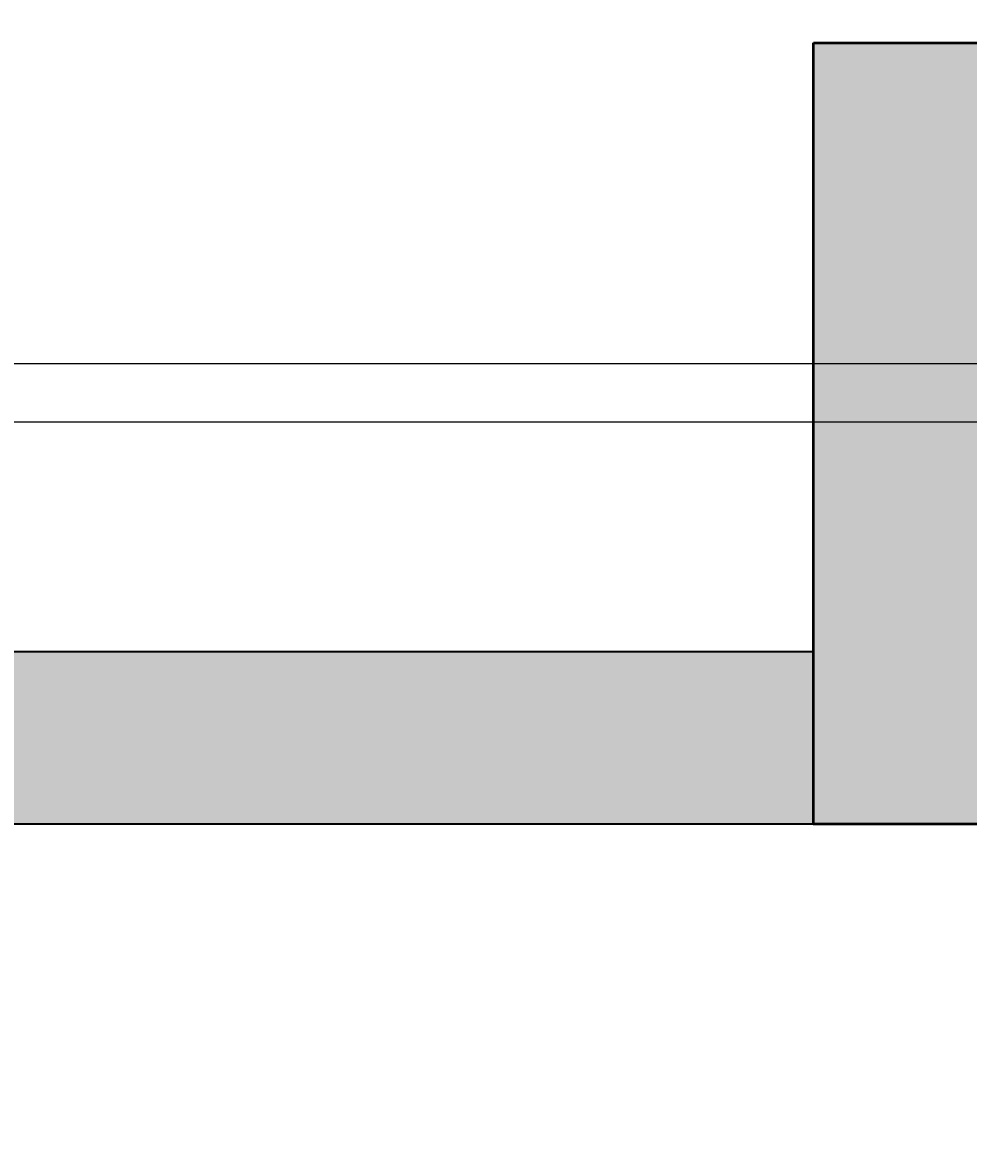
# Model space of a CAD drawing. Units: inches. Extents: x 1998 to 2588, y 1139 to 1977.
# Tile 19 of 134: x 2195 to 2220, y 1576 to 1605. Entities that reach past the tile are written whole.
import ezdxf

# ---------------------------------------------------------------- set-up
doc = ezdxf.new("R2010")
doc.units = ezdxf.units.IN
for name, color, linetype, lineweight in [('A-ANNO-DIMS', 2, 'Continuous', 18), ('A-COLS-PATT', 250, 'Continuous', 13), ('A-WALL-PATT', 252, 'Continuous', 13), ('COLUMN', 10, 'Continuous', 50), ('WALL', 200, 'Continuous', 35)]:
    doc.layers.add(name, color=color, linetype=linetype, lineweight=lineweight)
doc.styles.get("Standard").update_dxf_attribs({"font": 'arial.ttf'})
doc.dimstyles.get("Standard").update_dxf_attribs({"dimtxt": 0.18, "dimasz": 0.18, "dimexe": 0.18, "dimexo": 0.0625, "dimgap": 0.09, "dimtad": 0, "dimtih": 1, "dimtoh": 1, "dimdec": 4, "dimzin": 0, "dimdsep": 46, "dimtxsty": 'Standard', "dimcen": 0.09, "dimadec": 0, "dimazin": 0, "dimtfac": 1, "dimtdec": 4, "dimtofl": 0, "dimtmove": 0, "dimatfit": 3, "dimfxl": 1, "dimtolj": 1, "dimtzin": 0, "dimarcsym": 0})

# ---------------------------------------------------------------- blocks, each defined once
blk = doc.blocks.new('*D30')
at = {"layer": 'A-ANNO-DIMS', "color": 0, "lineweight": -2, "transparency": 16777216}
for p, q in [((2407.91, 1636.732), (1997.843, 1636.732)), ((1998.023, 1636.552), (1998.023, 1615.913)), ((1998.023, 1594.912), (1998.023, 1615.552)), ((2407.91, 1594.732), (1997.843, 1594.732))]:
    blk.add_line(p, q, dxfattribs=at)
at = {"layer": 'A-ANNO-DIMS', "color": 0, "transparency": 16777216}
for points in [[(1997.993, 1636.552), (1998.053, 1636.552), (1998.023, 1636.732)], [(1997.993, 1594.912), (1998.053, 1594.912), (1998.023, 1594.732)]]:
    blk.add_solid(points, dxfattribs=at)
at = {"layer": 'Defpoints', "color": 0, "transparency": 16777216}
for p in [(1998.023, 1636.732), (2407.973, 1636.732), (2407.973, 1594.732)]:
    blk.add_point(p, dxfattribs=at)
at = {"layer": 'A-ANNO-DIMS', "color": 0, "transparency": 16777216, "insert": (1998.023, 1615.732), "char_height": 0.18, "attachment_point": 5}
blk.add_mtext('\\A1;42', dxfattribs=at)
blk = doc.blocks.new('*D34')
at = {"layer": 'A-ANNO-DIMS', "color": 0, "lineweight": -2, "transparency": 16777216}
for p, q in [((2407.91, 1594.732), (1997.843, 1594.732)), ((1998.023, 1594.552), (1998.023, 1558.913)), ((1998.023, 1522.912), (1998.023, 1558.552)), ((2407.91, 1522.732), (1997.843, 1522.732))]:
    blk.add_line(p, q, dxfattribs=at)
at = {"layer": 'A-ANNO-DIMS', "color": 0, "transparency": 16777216}
for points in [[(1997.993, 1594.552), (1998.053, 1594.552), (1998.023, 1594.732)], [(1997.993, 1522.912), (1998.053, 1522.912), (1998.023, 1522.732)]]:
    blk.add_solid(points, dxfattribs=at)
at = {"layer": 'Defpoints', "color": 0, "transparency": 16777216}
for p in [(1998.023, 1594.732), (2407.973, 1594.732), (2407.973, 1522.732)]:
    blk.add_point(p, dxfattribs=at)
at = {"layer": 'A-ANNO-DIMS', "color": 0, "transparency": 16777216, "insert": (1998.023, 1558.732), "char_height": 0.18, "attachment_point": 5}
blk.add_mtext('\\A1;72', dxfattribs=at)
blk = doc.blocks.new('*D39')
at = {"layer": 'A-ANNO-DIMS', "color": 0, "lineweight": -2, "transparency": 16777216}
for p, q in [((2115.035, 1628.742), (2588.309, 1628.742)), ((2588.129, 1628.562), (2588.129, 1612.685)), ((2588.129, 1596.444), (2588.129, 1612.321)), ((2115.035, 1596.264), (2588.309, 1596.264))]:
    blk.add_line(p, q, dxfattribs=at)
at = {"layer": 'A-ANNO-DIMS', "color": 0, "transparency": 16777216}
for points in [[(2588.099, 1628.562), (2588.159, 1628.562), (2588.129, 1628.742)], [(2588.099, 1596.444), (2588.159, 1596.444), (2588.129, 1596.264)]]:
    blk.add_solid(points, dxfattribs=at)
at = {"layer": 'Defpoints', "color": 0, "transparency": 16777216}
for p in [(2114.973, 1628.742), (2588.129, 1628.742), (2114.973, 1596.264)]:
    blk.add_point(p, dxfattribs=at)
at = {"layer": 'A-ANNO-DIMS', "color": 0, "transparency": 16777216, "insert": (2588.129, 1612.503), "char_height": 0.18, "attachment_point": 5}
blk.add_mtext('\\A1;32.48', dxfattribs=at)

msp = doc.modelspace()

# ---------------------------------------------------------------- hatches: boundary and pattern name
at = {"layer": 'A-COLS-PATT'}
h = msp.add_hatch(color=256, dxfattribs=at)
h.dxf.hatch_style = 1
h.paths.add_polyline_path([(2099.4125, 1888.7324), (2087.9729, 1888.7324), (2087.9729, 1868.3278), (2099.4125, 1868.3278)])
h.paths.add_polyline_path([(2234.4125, 1888.7324), (2222.9729, 1888.7324), (2222.9729, 1868.3278), (2234.4125, 1868.3278)])
h.paths.add_polyline_path([(2341.4729, 1886.637), (2330.0332, 1886.637), (2330.0332, 1866.2324), (2341.4729, 1866.2324)])
h.paths.add_polyline_path([(2507.8006, 1882.7324), (2487.396, 1882.7324), (2487.396, 1871.2927), (2507.8006, 1871.2927)])
h.paths.add_polyline_path([(2510.9729, 1766.672), (2490.5682, 1766.672), (2490.5682, 1755.2324), (2510.9729, 1755.2324)])
h.paths.add_polyline_path([(2345.9729, 1759.7324), (2334.5332, 1759.7324), (2334.5332, 1739.3278), (2345.9729, 1739.3278)])
h.paths.add_polyline_path([(2234.4125, 1774.3318), (2222.9729, 1774.3318), (2222.9729, 1753.9272), (2234.4125, 1753.9272)])
h.paths.add_polyline_path([(2099.4125, 1775.637), (2087.9729, 1775.637), (2087.9729, 1755.2324), (2099.4125, 1755.2324)])
h.paths.add_polyline_path([(2098.0956, 1593.7241), (2077.691, 1593.7241), (2077.691, 1582.2845), (2098.0956, 1582.2845)])
h.paths.add_polyline_path([(2227.4729, 1604.637), (2216.0332, 1604.637), (2216.0332, 1584.2324), (2227.4729, 1584.2324)])
h.paths.add_polyline_path([(2345.9729, 1647.5211), (2334.5332, 1647.5211), (2334.5332, 1627.1165), (2345.9729, 1627.1165)])
h.paths.add_polyline_path([(2522.3775, 1641.2324), (2501.9729, 1641.2324), (2501.9729, 1629.7927), (2522.3775, 1629.7927)])
h.paths.add_polyline_path([(2522.3775, 1480.7324), (2501.9729, 1480.7324), (2501.9729, 1469.2927), (2522.3775, 1469.2927)])
h.paths.add_polyline_path([(2345.9729, 1488.5616), (2334.5332, 1488.5616), (2334.5332, 1468.1569), (2345.9729, 1468.1569)])
h.paths.add_polyline_path([(2234.4125, 1486.137), (2227.4729, 1486.137), (2227.4729, 1465.7324), (2234.4125, 1465.7324)])
h.paths.add_polyline_path([(2227.4729, 1486.137), (2222.9729, 1486.137), (2222.9729, 1465.7324), (2227.4729, 1465.7324)])
h.paths.add_polyline_path([(2108.3775, 1470.2324), (2087.9729, 1470.2324), (2087.9729, 1458.7927), (2108.3775, 1458.7927)])
h.paths.add_polyline_path([(2096.9729, 1365.5012), (2087.9729, 1365.5012), (2087.9729, 1345.0966), (2096.9729, 1345.0966)])
h.paths.add_polyline_path([(2087.9729, 1365.5012), (2085.5332, 1365.5012), (2085.5332, 1345.0966), (2087.9729, 1345.0966)])
h.paths.add_polyline_path([(2234.4125, 1285.137), (2222.9729, 1285.137), (2222.9729, 1264.7324), (2234.4125, 1264.7324)])
h.paths.add_polyline_path([(2345.9729, 1285.137), (2334.5332, 1285.137), (2334.5332, 1264.7324), (2345.9729, 1264.7324)])
h.paths.add_polyline_path([(2503.1458, 1240.172), (2482.7412, 1240.172), (2482.7412, 1228.7324), (2503.1458, 1228.7324)])
h.paths.add_polyline_path([(2510.9729, 1369.172), (2490.5682, 1369.172), (2490.5682, 1357.7324), (2510.9729, 1357.7324)])
at = {"layer": 'A-WALL-PATT'}
h = msp.add_hatch(color=256, dxfattribs=at)
h.dxf.hatch_style = 1
h.paths.add_polyline_path([(2222.9729, 1888.7324), (2099.4125, 1888.7324), (2099.4125, 1879.7324), (2222.9729, 1879.7324)])
h.paths.add_polyline_path([(2096.9729, 1868.3278), (2087.9729, 1868.3278), (2087.9729, 1775.637), (2096.9729, 1775.637)])
h.paths.add_polyline_path([(2227.4729, 1868.3278), (2222.9729, 1868.3278), (2222.9729, 1774.3318), (2227.4729, 1774.3318)])
h.paths.add_polyline_path([(2188.3019, 1759.7324), (2138.6074, 1759.7324), (2099.4125, 1759.7324), (2099.4125, 1755.2324), (2176.9729, 1755.2324), (2188.3019, 1755.2324)])
h.paths.add_polyline_path([(2087.9729, 1759.7324), (2059.4729, 1759.7324), (2059.4729, 1702.7324), (2087.9729, 1702.7324), (2087.9729, 1707.2324), (2063.9729, 1707.2324), (2063.9729, 1755.2324), (2087.9729, 1755.2324)])
h.paths.add_polyline_path([(2096.9729, 1755.2324), (2087.9729, 1755.2324), (2087.9729, 1707.2324), (2096.9729, 1707.2324)])
h.paths.add_polyline_path([(2187.0461, 1707.2324), (2105.9729, 1707.2324), (2096.9729, 1707.2324), (2087.9729, 1707.2324), (2087.9729, 1702.7324), (2105.9729, 1702.7324), (2114.9729, 1702.7324), (2187.0461, 1702.7324)])
h.paths.add_polyline_path([(2181.4729, 1719.2028), (2176.9729, 1719.2028), (2176.9729, 1707.2324), (2181.4729, 1707.2324)])
h.paths.add_polyline_path([(2216.0332, 1588.7324), (2114.9729, 1588.7324), (2105.9729, 1588.7324), (2105.9729, 1584.2324), (2216.0332, 1584.2324)])
h.paths.add_polyline_path([(2077.691, 1588.7324), (2061.4729, 1588.7324), (2061.4729, 1584.2324), (2077.691, 1584.2324)])
h.paths.add_polyline_path([(2105.9729, 1588.7324), (2098.0956, 1588.7324), (2098.0956, 1584.2324), (2105.9729, 1584.2324)])
h.paths.add_polyline_path([(2114.9729, 1596.2642), (2110.1012, 1596.2642), (2105.9729, 1596.2642), (2105.9729, 1588.7324), (2114.9729, 1588.7324)])
h.paths.add_polyline_path([(2114.9729, 1584.2324), (2105.9729, 1584.2324), (2105.9729, 1580.249), (2110.1012, 1580.249), (2114.9729, 1580.249)])
h.paths.add_polyline_path([(2114.9729, 1547.7716), (2110.1012, 1547.7716, -0.0318759), (2105.9729, 1548.035), (2105.9729, 1470.2324), (2108.3775, 1470.2324), (2108.3775, 1465.7324), (2186.2943, 1465.7324), (2186.2943, 1470.2324), (2114.9729, 1470.2324)])
h.paths.add_polyline_path([(2227.4729, 1584.2324), (2222.9729, 1584.2324), (2222.9729, 1486.137), (2227.4729, 1486.137)])
h.paths.add_polyline_path([(2295.4138, 1593.2324), (2227.4729, 1593.2324), (2227.4729, 1588.7324), (2295.4138, 1588.7324), (2295.4138, 1591.8729)])
h.paths.add_polyline_path([(2345.9729, 1627.1165), (2341.4729, 1627.1165), (2341.4729, 1593.2324), (2337.2869, 1593.2324), (2337.2869, 1591.8729), (2337.2869, 1588.7324), (2345.9729, 1588.7324)])
h.paths.add_polyline_path([(2291.9729, 1588.7324), (2287.4729, 1588.7324), (2287.4729, 1522.7324), (2291.9729, 1522.7324)])
h.paths.add_polyline_path([(2291.9729, 1522.7324), (2287.4729, 1522.7324), (2227.4729, 1522.7324), (2227.4729, 1518.2324), (2291.9729, 1518.2324)])
h.paths.add_polyline_path([(2295.7347, 1519.5919), (2295.7347, 1522.7324), (2291.9729, 1522.7324), (2291.9729, 1518.2324), (2295.7347, 1518.2324)])
h.paths.add_polyline_path([(2345.9729, 1522.7324), (2337.6078, 1522.7324), (2337.6078, 1519.5919), (2337.6078, 1518.2324), (2341.4729, 1518.2324), (2341.4729, 1488.5616), (2345.9729, 1488.5616)])
h.paths.add_polyline_path([(2345.9729, 1468.1569), (2341.4729, 1468.1569), (2341.4729, 1374.2324), (2227.4729, 1374.2324), (2227.4729, 1369.7324), (2345.9729, 1369.7324)])
h.paths.add_polyline_path([(2345.9729, 1369.7324), (2341.4729, 1369.7324), (2341.4729, 1362.2324), (2345.9729, 1362.2324)])
h.paths.add_polyline_path([(2345.9729, 1317.7324), (2345.9729, 1322.2324), (2341.4729, 1322.2324), (2341.4729, 1285.137), (2345.9729, 1285.137)], flags=17)
h.paths.add_polyline_path([(2356.2096, 1322.2324), (2345.9729, 1322.2324), (2345.9729, 1317.7324), (2356.2096, 1317.7324), (2356.2096, 1319.3088)], flags=17)
h.paths.add_polyline_path([(2393.9729, 1322.2324), (2375.6999, 1322.2324), (2375.6999, 1319.3088, -0.0202458), (2375.636, 1317.7324), (2393.9729, 1317.7324)], flags=17)
h.paths.add_polyline_path([(2398.4729, 1322.2324), (2393.9729, 1322.2324), (2393.9729, 1317.7324), (2393.9729, 1237.7324), (2345.9729, 1237.7324), (2345.9729, 1264.7324), (2341.4729, 1264.7324), (2341.4729, 1228.7324), (2393.9729, 1228.7324), (2482.7412, 1228.7324), (2482.7412, 1237.7324), (2398.4729, 1237.7324), (2398.4729, 1297.1029)])
h.paths.add_polyline_path([(2398.4729, 1362.2324), (2393.9729, 1362.2324), (2393.9729, 1357.7324), (2398.4729, 1357.7324)])
h.paths.add_polyline_path([(2345.9729, 1329.7549), (2341.4729, 1329.7549), (2341.4729, 1322.2324), (2345.9729, 1322.2324)])

# ---------------------------------------------------------------- linework, layer by layer
at = {"layer": 'COLUMN'}
msp.add_lwpolyline([(2216.0332, 1604.637), (2227.4729, 1604.637), (2227.4729, 1584.2324), (2216.0332, 1584.2324)], close=True, dxfattribs=at)
at = {"layer": 'WALL'}
for p, q in [((2216.0332, 1588.7324), (2114.9729, 1588.7324)), ((2227.4729, 1584.2324), (2105.9729, 1584.2324))]:
    msp.add_line(p, q, dxfattribs=at)

# ---------------------------------------------------------------- dimensions: what is measured, and where the dimension line sits
at = {"layer": 'A-ANNO-DIMS'}
for base, p1, p2, override, picture, middle in [((1998.0229, 1636.7324), (2407.9729, 1594.7324), (2407.9729, 1636.7324), {"dimdec": 0, "dimlfac": 1, "dimrnd": 0, "dimzin": 0, "dimdsep": 46, "dimlunit": 2}, '*D30', (1998.0229, 1615.7324)), ((2588.1286, 1628.7416), (2114.9729, 1596.2642), (2114.9729, 1628.7416), {"dimdec": 2, "dimlfac": 1, "dimrnd": 0, "dimzin": 0, "dimdsep": 46, "dimlunit": 2}, '*D39', (2588.1286, 1612.5029)), ((1998.0229, 1594.7324), (2407.9729, 1522.7324), (2407.9729, 1594.7324), {"dimdec": 0, "dimlfac": 1, "dimrnd": 0, "dimzin": 0, "dimdsep": 46, "dimlunit": 2}, '*D34', (1998.0229, 1558.7324))]:
    dim = msp.add_linear_dim(base=base, p1=p1, p2=p2, angle=90, dimstyle='Standard', override=override, dxfattribs=at)
    dim.commit()
    dim.dimension.update_dxf_attribs({"geometry": picture, "text_midpoint": middle})

doc.saveas('drawing.dxf')
